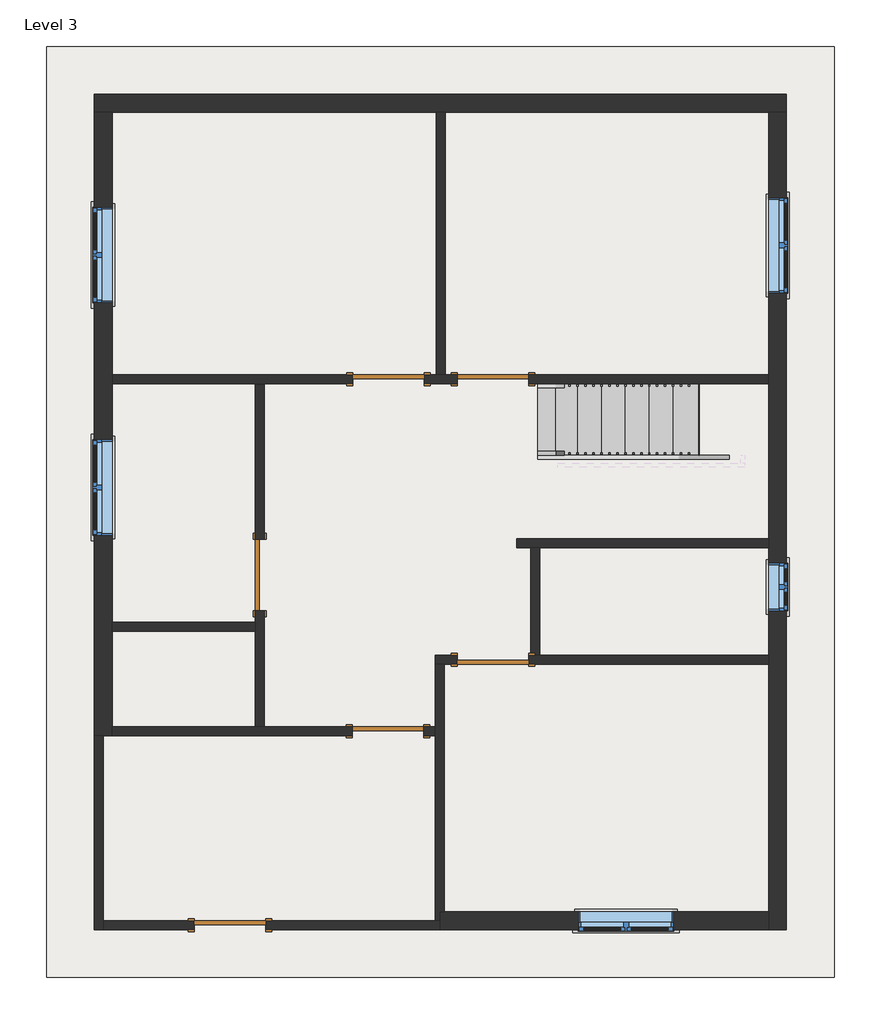
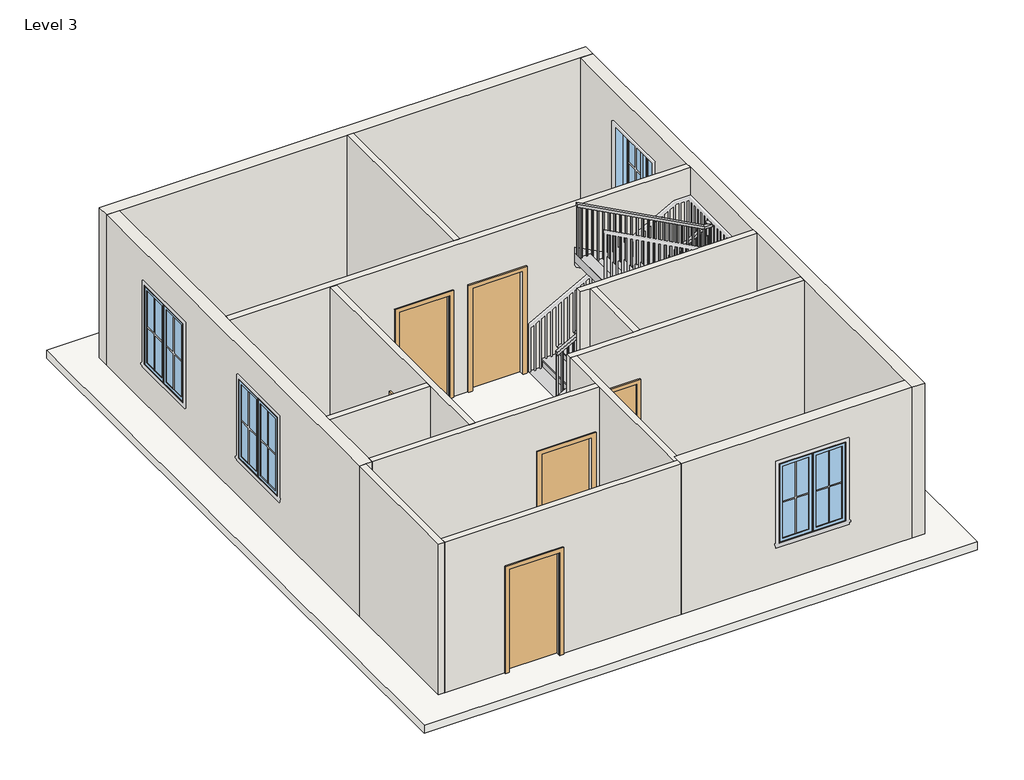
# One storey, part 1 of 2: 15 walls, 6 doors, 5 windows, 1 railing, 1 roof, 1 stair flight.
"""IFC4 building model written with IfcOpenShell, lengths in millimetres."""

from ifc_helpers import new_model, si_unit, frame, origin, place, context, project, spatial, polyline, outline, extrude, faceted_brep, transform, mapped, element, save
from components import door_305aa2a5, door_e5f9f3c4, stair_flight_a6cfe23b, window_c417fced, window_8377141f

model = new_model("IFC4")

# Units and contexts
model_context = context("Model", 3, world=origin())
ifc_project = project(units=[si_unit("LENGTHUNIT", "METRE", prefix="MILLI")], contexts=[model_context])

# Site, building, storey
site = spatial("IfcSite", under=ifc_project)
building = spatial("IfcBuilding", under=site)
storey = spatial("IfcBuildingStorey", under=building, Name="Level 3", Elevation=6096.0)

# Doors
placement = place(None, origin())
door_shape = door_305aa2a5(model_context)
element("IfcDoor", 1, ObjectType="Single-Flush : 36\" x 84\"", at=placement, inside=storey, context=model_context, shape_type="MappedRepresentation", body=[
    mapped(door_shape, transform((8001.0, 9251.95, 6096.0), x_axis=(-1.0, 0.0, 0.0), y_axis=(0.0, -1.0, 0.0), z_axis=(0.0, 0.0, 1.0))),
])
element("IfcDoor", 2, ObjectType="Single-Flush : 36\" x 84\"", at=placement, inside=storey, context=model_context, shape_type="MappedRepresentation", body=[
    mapped(door_shape, transform((5022.9818578, 6750.05, 6096.0), x_axis=(0.0, -1.0, 0.0), y_axis=(1.0, 0.0, 0.0), z_axis=(0.0, 0.0, 1.0))),
])
door_2_shape = door_e5f9f3c4(model_context)
element("IfcDoor", 3, ObjectType="Single-Flush : 36\" x 84\"", at=placement, inside=storey, context=model_context, shape_type="MappedRepresentation", body=[
    mapped(door_2_shape, transform((6667.5, 9251.95, 6096.0), x_axis=(1.0, 0.0, 0.0), y_axis=(0.0, 1.0, 0.0), z_axis=(0.0, 0.0, 1.0))),
])
element("IfcDoor", 4, ObjectType="Single-Flush : 36\" x 84\"", at=placement, inside=storey, context=model_context, shape_type="MappedRepresentation", body=[
    mapped(door_2_shape, transform((8001.0, 5670.55, 6096.0), x_axis=(-1.0, 0.0, 0.0), y_axis=(0.0, -1.0, 0.0), z_axis=(0.0, 0.0, 1.0))),
])
element("IfcDoor", 5, ObjectType="Single-Flush : 36\" x 84\"", at=placement, inside=storey, context=model_context, shape_type="MappedRepresentation", body=[
    mapped(door_2_shape, transform((6658.76875, 4756.15, 6096.0), x_axis=(1.0, 0.0, 0.0), y_axis=(0.0, 1.0, 0.0), z_axis=(0.0, 0.0, 1.0))),
])
element("IfcDoor", 6, ObjectType="Single-Flush : 36\" x 84\"", at=placement, inside=storey, context=model_context, shape_type="MappedRepresentation", body=[
    mapped(door_2_shape, transform((4641.85, 2279.65, 6096.0), x_axis=(1.0, 0.0, 0.0), y_axis=(0.0, 1.0, 0.0), z_axis=(0.0, 0.0, 1.0))),
])

# Railing
element("IfcRailing", 7, ObjectType="Handrail - Rectangular", at=placement, inside=storey, context=model_context, shape_type="SolidModel", body=[
    faceted_brep([(8572.5, 8331.2, 7170.8210526), (8572.5, 8331.2, 7112.9285199), (8572.5, 8280.4, 7112.9285199), (8572.5, 8280.4, 7170.8210526), (11137.9, 8331.2, 8572.962753), (11188.7, 8331.2, 8542.8354025), (11188.7, 8280.4, 8542.8354025), (11137.9, 8280.4, 8572.962753), (11137.9, 8331.2, 8614.6105263), (11188.7, 8331.2, 8563.8105263), (11188.7, 8280.4, 8563.8105263), (11137.9, 8280.4, 8614.6105263), (11264.9, 8331.2, 8614.6105263), (11264.9, 8331.2, 8563.8105263), (11214.1, 8280.4, 8563.8105263), (11214.1, 8280.4, 8614.6105263), (11264.9, 8204.2, 8614.6105263), (11264.9, 8153.4, 8563.8105263), (11214.1, 8153.4, 8563.8105263), (11214.1, 8204.2, 8614.6105263), (11264.9, 8204.2, 8815.9901456), (11264.9, 8153.4, 8765.1901456), (11214.1, 8153.4, 8765.1901456), (11214.1, 8204.2, 8815.9901456), (11264.9, 8077.2, 8815.9901456), (11264.9, 8077.2, 8765.1901456), (11214.1, 8128.0, 8765.1901456), (11214.1, 8128.0, 8815.9901456), (11137.9, 8077.2, 8815.9901456), (11125.1122768, 8077.2, 8765.1901456), (11125.1122768, 8128.0, 8765.1901456), (11137.9, 8128.0, 8815.9901456), (8826.5, 8077.2, 10058.4), (8826.5, 8128.0, 10058.4), (8826.5, 8128.0, 10000.7264198), (8826.5, 8077.2, 10000.7264198)], [[[0, 1, 2, 3]], [[1, 0, 4, 5]], [[2, 1, 5, 6]], [[3, 2, 6, 7]], [[0, 3, 7, 4]], [[5, 4, 8, 9]], [[6, 5, 9, 10]], [[7, 6, 10, 11]], [[4, 7, 11, 8]], [[9, 8, 12, 13]], [[10, 9, 13, 14]], [[11, 10, 14, 15]], [[8, 11, 15, 12]], [[13, 12, 16, 17]], [[14, 13, 17, 18]], [[15, 14, 18, 19]], [[12, 15, 19, 16]], [[17, 16, 20, 21]], [[18, 17, 21, 22]], [[19, 18, 22, 23]], [[16, 19, 23, 20]], [[21, 20, 24, 25]], [[22, 21, 25, 26]], [[23, 22, 26, 27]], [[20, 23, 27, 24]], [[25, 24, 28, 29]], [[26, 25, 29, 30]], [[27, 26, 30, 31]], [[24, 27, 31, 28]], [[32, 33, 34, 35]], [[29, 28, 32, 35]], [[30, 29, 35, 34]], [[31, 30, 34, 33]], [[28, 31, 33, 32]]]),
    extrude(outline(polyline([(9954.6480323, 8912.225), (9964.887674, 8893.175), (8983.5789474, 8893.175), (8983.5789474, 8912.225), (9954.6480323, 8912.225)])), frame((0.0, 8093.075, 0.0), z_axis=(0.0, 1.0, 0.0), x_axis=(0.0, 0.0, 1.0)), (0.0, 0.0, 1.0), 19.05),
    extrude(outline(polyline([(9900.0366101, 9013.825), (9910.2762518, 8994.775), (8983.5789474, 8994.775), (8983.5789474, 9013.825), (9900.0366101, 9013.825)])), frame((0.0, 8093.075, 0.0), z_axis=(0.0, 1.0, 0.0), x_axis=(0.0, 0.0, 1.0)), (0.0, 0.0, 1.0), 19.05),
    extrude(outline(polyline([(9845.425188, 9115.425), (9855.6648296, 9096.375), (8823.1578947, 9096.375), (8823.1578947, 9115.425), (9845.425188, 9115.425)])), frame((0.0, 8093.075, 0.0), z_axis=(0.0, 1.0, 0.0), x_axis=(0.0, 0.0, 1.0)), (0.0, 0.0, 1.0), 19.05),
    extrude(outline(polyline([(9790.8137658, 9217.025), (9801.0534074, 9197.975), (8823.1578947, 9197.975), (8823.1578947, 9217.025), (9790.8137658, 9217.025)])), frame((0.0, 8093.075, 0.0), z_axis=(0.0, 1.0, 0.0), x_axis=(0.0, 0.0, 1.0)), (0.0, 0.0, 1.0), 19.05),
    extrude(outline(polyline([(9736.1597952, 9318.625), (9746.5717386, 9299.575), (8823.1578947, 9299.575), (8823.1578947, 9318.625), (9736.1597952, 9318.625)])), frame((0.0, 8093.075, 0.0), z_axis=(0.0, 1.0, 0.0), x_axis=(0.0, 0.0, 1.0)), (0.0, 0.0, 1.0), 19.05),
    extrude(outline(polyline([(9681.5909214, 9420.225), (9691.8305631, 9401.175), (8662.7368421, 9401.175), (8662.7368421, 9420.225), (9681.5909214, 9420.225)])), frame((0.0, 8093.075, 0.0), z_axis=(0.0, 1.0, 0.0), x_axis=(0.0, 0.0, 1.0)), (0.0, 0.0, 1.0), 19.05),
    extrude(outline(polyline([(9626.9794993, 9521.825), (9637.2191409, 9502.775), (8662.7368421, 9502.775), (8662.7368421, 9521.825), (9626.9794993, 9521.825)])), frame((0.0, 8093.075, 0.0), z_axis=(0.0, 1.0, 0.0), x_axis=(0.0, 0.0, 1.0)), (0.0, 0.0, 1.0), 19.05),
    extrude(outline(polyline([(9572.3680771, 9623.425), (9582.6077187, 9604.375), (8662.7368421, 9604.375), (8662.7368421, 9623.425), (9572.3680771, 9623.425)])), frame((0.0, 8093.075, 0.0), z_axis=(0.0, 1.0, 0.0), x_axis=(0.0, 0.0, 1.0)), (0.0, 0.0, 1.0), 19.05),
    extrude(outline(polyline([(9517.7566549, 9725.025), (9527.9962966, 9705.975), (8502.3157895, 9705.975), (8502.3157895, 9725.025), (9517.7566549, 9725.025)])), frame((0.0, 8093.075, 0.0), z_axis=(0.0, 1.0, 0.0), x_axis=(0.0, 0.0, 1.0)), (0.0, 0.0, 1.0), 19.05),
    extrude(outline(polyline([(9463.1452327, 9826.625), (9473.3848744, 9807.575), (8502.3157895, 9807.575), (8502.3157895, 9826.625), (9463.1452327, 9826.625)])), frame((0.0, 8093.075, 0.0), z_axis=(0.0, 1.0, 0.0), x_axis=(0.0, 0.0, 1.0)), (0.0, 0.0, 1.0), 19.05),
    extrude(outline(polyline([(9408.5338106, 9928.225), (9418.7734522, 9909.175), (8502.3157895, 9909.175), (8502.3157895, 9928.225), (9408.5338106, 9928.225)])), frame((0.0, 8093.075, 0.0), z_axis=(0.0, 1.0, 0.0), x_axis=(0.0, 0.0, 1.0)), (0.0, 0.0, 1.0), 19.05),
    extrude(outline(polyline([(9353.9223884, 10029.825), (9364.1620301, 10010.775), (8341.8947368, 10010.775), (8341.8947368, 10029.825), (9353.9223884, 10029.825)])), frame((0.0, 8093.075, 0.0), z_axis=(0.0, 1.0, 0.0), x_axis=(0.0, 0.0, 1.0)), (0.0, 0.0, 1.0), 19.05),
    extrude(outline(polyline([(9299.3109662, 10131.425), (9309.5506079, 10112.375), (8341.8947368, 10112.375), (8341.8947368, 10131.425), (9299.3109662, 10131.425)])), frame((0.0, 8093.075, 0.0), z_axis=(0.0, 1.0, 0.0), x_axis=(0.0, 0.0, 1.0)), (0.0, 0.0, 1.0), 19.05),
    extrude(outline(polyline([(9244.6995441, 10233.025), (9254.9391857, 10213.975), (8341.8947368, 10213.975), (8341.8947368, 10233.025), (9244.6995441, 10233.025)])), frame((0.0, 8093.075, 0.0), z_axis=(0.0, 1.0, 0.0), x_axis=(0.0, 0.0, 1.0)), (0.0, 0.0, 1.0), 19.05),
    extrude(outline(polyline([(9190.0881219, 10334.625), (9200.3277635, 10315.575), (8181.4736842, 10315.575), (8181.4736842, 10334.625), (9190.0881219, 10334.625)])), frame((0.0, 8093.075, 0.0), z_axis=(0.0, 1.0, 0.0), x_axis=(0.0, 0.0, 1.0)), (0.0, 0.0, 1.0), 19.05),
    extrude(outline(polyline([(9135.4766997, 10436.225), (9145.7163414, 10417.175), (8181.4736842, 10417.175), (8181.4736842, 10436.225), (9135.4766997, 10436.225)])), frame((0.0, 8093.075, 0.0), z_axis=(0.0, 1.0, 0.0), x_axis=(0.0, 0.0, 1.0)), (0.0, 0.0, 1.0), 19.05),
    extrude(outline(polyline([(9080.8652775, 10537.825), (9091.1049192, 10518.775), (8181.4736842, 10518.775), (8181.4736842, 10537.825), (9080.8652775, 10537.825)])), frame((0.0, 8093.075, 0.0), z_axis=(0.0, 1.0, 0.0), x_axis=(0.0, 0.0, 1.0)), (0.0, 0.0, 1.0), 19.05),
    extrude(outline(polyline([(9026.2538554, 10639.425), (9036.493497, 10620.375), (8021.0526316, 10620.375), (8021.0526316, 10639.425), (9026.2538554, 10639.425)])), frame((0.0, 8093.075, 0.0), z_axis=(0.0, 1.0, 0.0), x_axis=(0.0, 0.0, 1.0)), (0.0, 0.0, 1.0), 19.05),
    extrude(outline(polyline([(8971.6424332, 10741.025), (8981.8820749, 10721.975), (8021.0526316, 10721.975), (8021.0526316, 10741.025), (8971.6424332, 10741.025)])), frame((0.0, 8093.075, 0.0), z_axis=(0.0, 1.0, 0.0), x_axis=(0.0, 0.0, 1.0)), (0.0, 0.0, 1.0), 19.05),
    extrude(outline(polyline([(8917.031011, 10842.625), (8927.2706527, 10823.575), (8021.0526316, 10823.575), (8021.0526316, 10842.625), (8917.031011, 10842.625)])), frame((0.0, 8093.075, 0.0), z_axis=(0.0, 1.0, 0.0), x_axis=(0.0, 0.0, 1.0)), (0.0, 0.0, 1.0), 19.05),
    extrude(outline(polyline([(8862.4195889, 10944.225), (8872.6592305, 10925.175), (7860.6315789, 10925.175), (7860.6315789, 10944.225), (8862.4195889, 10944.225)])), frame((0.0, 8093.075, 0.0), z_axis=(0.0, 1.0, 0.0), x_axis=(0.0, 0.0, 1.0)), (0.0, 0.0, 1.0), 19.05),
    extrude(outline(polyline([(8807.8081667, 11045.825), (8818.0478083, 11026.775), (7860.6315789, 11026.775), (7860.6315789, 11045.825), (8807.8081667, 11045.825)])), frame((0.0, 8093.075, 0.0), z_axis=(0.0, 1.0, 0.0), x_axis=(0.0, 0.0, 1.0)), (0.0, 0.0, 1.0), 19.05),
    extrude(outline(polyline([(8753.1967445, 11147.425), (8763.4363862, 11128.375), (7860.6315789, 11128.375), (7860.6315789, 11147.425), (8753.1967445, 11147.425)])), frame((0.0, 8093.075, 0.0), z_axis=(0.0, 1.0, 0.0), x_axis=(0.0, 0.0, 1.0)), (0.0, 0.0, 1.0), 19.05),
    extrude(outline(polyline([(11229.975, 8213.725), (11249.025, 8213.725), (11249.025, 8194.675), (11229.975, 8194.675), (11229.975, 8213.725)])), frame((0.0, 0.0, 7700.2105263), z_axis=(0.0, 0.0, 1.0), x_axis=(1.0, 0.0, 0.0)), (0.0, 0.0, 1.0), 863.6),
    extrude(outline(polyline([(11204.575, 8296.275), (11204.575, 8315.325), (11223.625, 8315.325), (11223.625, 8296.275), (11204.575, 8296.275)])), frame((0.0, 0.0, 7700.2105263), z_axis=(0.0, 0.0, 1.0), x_axis=(1.0, 0.0, 0.0)), (0.0, 0.0, 1.0), 863.6),
    extrude(outline(polyline([(8506.3936009, 11122.025), (8495.9816576, 11102.975), (7539.7894737, 11102.975), (7539.7894737, 11122.025), (8506.3936009, 11122.025)])), frame((0.0, 8296.275, 0.0), z_axis=(0.0, 1.0, 0.0), x_axis=(0.0, 0.0, 1.0)), (0.0, 0.0, 1.0), 19.05),
    extrude(outline(polyline([(8450.8632365, 11020.425), (8440.4512932, 11001.375), (7539.7894737, 11001.375), (7539.7894737, 11020.425), (8450.8632365, 11020.425)])), frame((0.0, 8296.275, 0.0), z_axis=(0.0, 1.0, 0.0), x_axis=(0.0, 0.0, 1.0)), (0.0, 0.0, 1.0), 19.05),
    extrude(outline(polyline([(8395.3328722, 10918.825), (8384.9209288, 10899.775), (7539.7894737, 10899.775), (7539.7894737, 10918.825), (8395.3328722, 10918.825)])), frame((0.0, 8296.275, 0.0), z_axis=(0.0, 1.0, 0.0), x_axis=(0.0, 0.0, 1.0)), (0.0, 0.0, 1.0), 19.05),
    extrude(outline(polyline([(8339.8025078, 10817.225), (8329.3905645, 10798.175), (7379.3684211, 10798.175), (7379.3684211, 10817.225), (8339.8025078, 10817.225)])), frame((0.0, 8296.275, 0.0), z_axis=(0.0, 1.0, 0.0), x_axis=(0.0, 0.0, 1.0)), (0.0, 0.0, 1.0), 19.05),
    extrude(outline(polyline([(8284.2721434, 10715.625), (8273.8602001, 10696.575), (7379.3684211, 10696.575), (7379.3684211, 10715.625), (8284.2721434, 10715.625)])), frame((0.0, 8296.275, 0.0), z_axis=(0.0, 1.0, 0.0), x_axis=(0.0, 0.0, 1.0)), (0.0, 0.0, 1.0), 19.05),
    extrude(outline(polyline([(8228.741779, 10614.025), (8218.3298357, 10594.975), (7379.3684211, 10594.975), (7379.3684211, 10614.025), (8228.741779, 10614.025)])), frame((0.0, 8296.275, 0.0), z_axis=(0.0, 1.0, 0.0), x_axis=(0.0, 0.0, 1.0)), (0.0, 0.0, 1.0), 19.05),
    extrude(outline(polyline([(8173.2114147, 10512.425), (8162.7994714, 10493.375), (7218.9473684, 10493.375), (7218.9473684, 10512.425), (8173.2114147, 10512.425)])), frame((0.0, 8296.275, 0.0), z_axis=(0.0, 1.0, 0.0), x_axis=(0.0, 0.0, 1.0)), (0.0, 0.0, 1.0), 19.05),
    extrude(outline(polyline([(8117.6810503, 10410.825), (8107.269107, 10391.775), (7218.9473684, 10391.775), (7218.9473684, 10410.825), (8117.6810503, 10410.825)])), frame((0.0, 8296.275, 0.0), z_axis=(0.0, 1.0, 0.0), x_axis=(0.0, 0.0, 1.0)), (0.0, 0.0, 1.0), 19.05),
    extrude(outline(polyline([(8062.1506859, 10309.225), (8051.7387426, 10290.175), (7218.9473684, 10290.175), (7218.9473684, 10309.225), (8062.1506859, 10309.225)])), frame((0.0, 8296.275, 0.0), z_axis=(0.0, 1.0, 0.0), x_axis=(0.0, 0.0, 1.0)), (0.0, 0.0, 1.0), 19.05),
    extrude(outline(polyline([(8006.6203216, 10207.625), (7996.2083782, 10188.575), (7058.5263158, 10188.575), (7058.5263158, 10207.625), (8006.6203216, 10207.625)])), frame((0.0, 8296.275, 0.0), z_axis=(0.0, 1.0, 0.0), x_axis=(0.0, 0.0, 1.0)), (0.0, 0.0, 1.0), 19.05),
    extrude(outline(polyline([(7951.0899572, 10106.025), (7940.6780139, 10086.975), (7058.5263158, 10086.975), (7058.5263158, 10106.025), (7951.0899572, 10106.025)])), frame((0.0, 8296.275, 0.0), z_axis=(0.0, 1.0, 0.0), x_axis=(0.0, 0.0, 1.0)), (0.0, 0.0, 1.0), 19.05),
    extrude(outline(polyline([(7895.5595928, 10004.425), (7885.1476495, 9985.375), (7058.5263158, 9985.375), (7058.5263158, 10004.425), (7895.5595928, 10004.425)])), frame((0.0, 8296.275, 0.0), z_axis=(0.0, 1.0, 0.0), x_axis=(0.0, 0.0, 1.0)), (0.0, 0.0, 1.0), 19.05),
    extrude(outline(polyline([(7840.0292284, 9902.825), (7829.6172851, 9883.775), (6898.1052632, 9883.775), (6898.1052632, 9902.825), (7840.0292284, 9902.825)])), frame((0.0, 8296.275, 0.0), z_axis=(0.0, 1.0, 0.0), x_axis=(0.0, 0.0, 1.0)), (0.0, 0.0, 1.0), 19.05),
    extrude(outline(polyline([(7784.4988641, 9801.225), (7774.0869207, 9782.175), (6898.1052632, 9782.175), (6898.1052632, 9801.225), (7784.4988641, 9801.225)])), frame((0.0, 8296.275, 0.0), z_axis=(0.0, 1.0, 0.0), x_axis=(0.0, 0.0, 1.0)), (0.0, 0.0, 1.0), 19.05),
    extrude(outline(polyline([(7728.9684997, 9699.625), (7718.5565564, 9680.575), (6898.1052632, 9680.575), (6898.1052632, 9699.625), (7728.9684997, 9699.625)])), frame((0.0, 8296.275, 0.0), z_axis=(0.0, 1.0, 0.0), x_axis=(0.0, 0.0, 1.0)), (0.0, 0.0, 1.0), 19.05),
    extrude(outline(polyline([(7673.4381353, 9598.025), (7663.026192, 9578.975), (6737.6842105, 9578.975), (6737.6842105, 9598.025), (7673.4381353, 9598.025)])), frame((0.0, 8296.275, 0.0), z_axis=(0.0, 1.0, 0.0), x_axis=(0.0, 0.0, 1.0)), (0.0, 0.0, 1.0), 19.05),
    extrude(outline(polyline([(7617.9077709, 9496.425), (7607.4958276, 9477.375), (6737.6842105, 9477.375), (6737.6842105, 9496.425), (7617.9077709, 9496.425)])), frame((0.0, 8296.275, 0.0), z_axis=(0.0, 1.0, 0.0), x_axis=(0.0, 0.0, 1.0)), (0.0, 0.0, 1.0), 19.05),
    extrude(outline(polyline([(7562.3774066, 9394.825), (7551.9654633, 9375.775), (6737.6842105, 9375.775), (6737.6842105, 9394.825), (7562.3774066, 9394.825)])), frame((0.0, 8296.275, 0.0), z_axis=(0.0, 1.0, 0.0), x_axis=(0.0, 0.0, 1.0)), (0.0, 0.0, 1.0), 19.05),
    extrude(outline(polyline([(7506.8470422, 9293.225), (7496.4350989, 9274.175), (6577.2631579, 9274.175), (6577.2631579, 9293.225), (7506.8470422, 9293.225)])), frame((0.0, 8296.275, 0.0), z_axis=(0.0, 1.0, 0.0), x_axis=(0.0, 0.0, 1.0)), (0.0, 0.0, 1.0), 19.05),
    extrude(outline(polyline([(7451.3166778, 9191.625), (7440.9047345, 9172.575), (6577.2631579, 9172.575), (6577.2631579, 9191.625), (7451.3166778, 9191.625)])), frame((0.0, 8296.275, 0.0), z_axis=(0.0, 1.0, 0.0), x_axis=(0.0, 0.0, 1.0)), (0.0, 0.0, 1.0), 19.05),
    extrude(outline(polyline([(7395.7863135, 9090.025), (7385.3743701, 9070.975), (6577.2631579, 9070.975), (6577.2631579, 9090.025), (7395.7863135, 9090.025)])), frame((0.0, 8296.275, 0.0), z_axis=(0.0, 1.0, 0.0), x_axis=(0.0, 0.0, 1.0)), (0.0, 0.0, 1.0), 19.05),
    extrude(outline(polyline([(7340.2559491, 8988.425), (7329.8440058, 8969.375), (6416.8421053, 8969.375), (6416.8421053, 8988.425), (7340.2559491, 8988.425)])), frame((0.0, 8296.275, 0.0), z_axis=(0.0, 1.0, 0.0), x_axis=(0.0, 0.0, 1.0)), (0.0, 0.0, 1.0), 19.05),
    extrude(outline(polyline([(7284.7255847, 8886.825), (7274.3136414, 8867.775), (6416.8421053, 8867.775), (6416.8421053, 8886.825), (7284.7255847, 8886.825)])), frame((0.0, 8296.275, 0.0), z_axis=(0.0, 1.0, 0.0), x_axis=(0.0, 0.0, 1.0)), (0.0, 0.0, 1.0), 19.05),
    extrude(outline(polyline([(7229.1952203, 8785.225), (7218.783277, 8766.175), (6256.4210526, 8766.175), (6256.4210526, 8785.225), (7229.1952203, 8785.225)])), frame((0.0, 8296.275, 0.0), z_axis=(0.0, 1.0, 0.0), x_axis=(0.0, 0.0, 1.0)), (0.0, 0.0, 1.0), 19.05),
    extrude(outline(polyline([(7173.664856, 8683.625), (7163.2529126, 8664.575), (6256.4210526, 8664.575), (6256.4210526, 8683.625), (7173.664856, 8683.625)])), frame((0.0, 8296.275, 0.0), z_axis=(0.0, 1.0, 0.0), x_axis=(0.0, 0.0, 1.0)), (0.0, 0.0, 1.0), 19.05),
    extrude(outline(polyline([(11229.975, 8112.125), (11249.025, 8112.125), (11249.025, 8093.075), (11229.975, 8093.075), (11229.975, 8112.125)])), frame((0.0, 0.0, 7700.2105263), z_axis=(0.0, 0.0, 1.0), x_axis=(1.0, 0.0, 0.0)), (0.0, 0.0, 1.0), 1064.9796193),
    extrude(outline(polyline([(11229.975, 8296.275), (11229.975, 8315.325), (11249.025, 8315.325), (11249.025, 8296.275), (11229.975, 8296.275)])), frame((0.0, 0.0, 7700.2105263), z_axis=(0.0, 0.0, 1.0), x_axis=(1.0, 0.0, 0.0)), (0.0, 0.0, 1.0), 863.6),
    extrude(outline(polyline([(9990.4867781, 8845.55), (10000.7264198, 8826.5), (8983.5789474, 8826.5), (8983.5789474, 8845.55), (9990.4867781, 8845.55)])), frame((0.0, 8093.075, 0.0), z_axis=(0.0, 1.0, 0.0), x_axis=(0.0, 0.0, 1.0)), (0.0, 0.0, 1.0), 19.05),
    extrude(outline(polyline([(7123.3404633, 8591.55), (7112.9285199, 8572.5), (6256.4210526, 8572.5), (6256.4210526, 8591.55), (7123.3404633, 8591.55)])), frame((0.0, 8296.275, 0.0), z_axis=(0.0, 1.0, 0.0), x_axis=(0.0, 0.0, 1.0)), (0.0, 0.0, 1.0), 19.05),
])

# Roof
element("IfcRoof", 8, ObjectType="Generic - 12\"", at=placement, inside=storey, context=model_context, shape_type="SweptSolid", body=[
    extrude(outline(polyline([(2298.7, 13500.1), (12357.1, 13500.1), (12357.1, 1612.9), (2298.7, 1612.9), (2298.7, 13500.1)])), frame((0.0, 0.0, 6096.0), z_axis=(0.0, 0.0, 1.0), x_axis=(1.0, 0.0, 0.0)), (0.0, 0.0, 1.0), 152.4),
])

# Stair flight
stair_flight_shape = stair_flight_a6cfe23b(model_context)
element("IfcStairFlight", 9, ObjectType="2\" Tread 1\" Nosing 1/4\" Riser", at=placement, inside=storey, context=model_context, shape_type="MappedRepresentation", body=[
    mapped(stair_flight_shape, transform((0.0, 0.0, 0.0), x_axis=(1.0, 0.0, 0.0), y_axis=(0.0, 1.0, 0.0), z_axis=(0.0, 0.0, 1.0))),
])

# Walls
element("IfcWall", 10, ObjectType="Generic - 5\"", at=placement, inside=storey, context=model_context, shape_type="Brep", body=[
    faceted_brep([(7115.96875, 4699.0, 8229.6), (7115.96875, 4699.0, 6096.0), (7264.4, 4699.0, 6096.0), (7264.4, 4699.0, 9144.0), (3136.9, 4699.0, 9144.0), (3136.9, 4699.0, 6096.0), (6201.56875, 4699.0, 6096.0), (6201.56875, 4699.0, 8229.6), (7264.4, 4813.3, 6096.0), (7115.96875, 4813.3, 6096.0), (7115.96875, 4813.3, 8229.6), (6201.56875, 4813.3, 8229.6), (6201.56875, 4813.3, 6096.0), (5080.1318578, 4813.3, 6096.0), (4965.8318578, 4813.3, 6096.0), (3136.9, 4813.3, 6096.0), (3136.9, 4813.3, 9144.0), (4965.8318578, 4813.3, 9144.0), (5080.1318578, 4813.3, 9144.0), (7264.4, 4813.3, 9144.0)], [[[0, 1, 2, 3, 4, 5, 6, 7]], [[8, 9, 10, 11, 12, 13, 14, 15, 16, 17, 18, 19]], [[6, 5, 15, 14, 13, 12]], [[2, 1, 9, 8]], [[4, 3, 19, 18, 17, 16]], [[5, 4, 16, 15]], [[3, 2, 8, 19]], [[10, 9, 1, 0]], [[11, 10, 0, 7]], [[12, 11, 7, 6]]]),
])
element("IfcWall", 11, ObjectType="Generic - 5\"", at=placement, inside=storey, context=model_context, shape_type="SweptSolid", body=[
    extrude(outline(polyline([(4965.8318578, 6032.5), (3136.9, 6032.5), (3136.9, 6146.8), (4965.8318578, 6146.8), (4965.8318578, 6032.5)])), frame((0.0, 0.0, 6096.0), z_axis=(0.0, 0.0, 1.0), x_axis=(1.0, 0.0, 0.0)), (0.0, 0.0, 1.0), 3048.0),
])
element("IfcWall", 12, ObjectType="Generic - 5\"", at=placement, inside=storey, context=model_context, shape_type="Brep", body=[
    faceted_brep([(5080.1318578, 4813.3, 6096.0), (5080.1318578, 6292.85, 6096.0), (5080.1318578, 6292.85, 8229.6), (5080.1318578, 7207.25, 8229.6), (5080.1318578, 7207.25, 6096.0), (5080.1318578, 9182.1, 6096.0), (5080.1318578, 9182.1, 9144.0), (5080.1318578, 4813.3, 9144.0), (4965.8318578, 6292.85, 8229.6), (4965.8318578, 6292.85, 6096.0), (4965.8318578, 6146.8, 6096.0), (4965.8318578, 6032.5, 6096.0), (4965.8318578, 4813.3, 6096.0), (4965.8318578, 4813.3, 9144.0), (4965.8318578, 6032.5, 9144.0), (4965.8318578, 6146.8, 9144.0), (4965.8318578, 9182.1, 9144.0), (4965.8318578, 9182.1, 6096.0), (4965.8318578, 7207.25, 6096.0), (4965.8318578, 7207.25, 8229.6)], [[[0, 1, 2, 3, 4, 5, 6, 7]], [[8, 9, 10, 11, 12, 13, 14, 15, 16, 17, 18, 19]], [[18, 17, 5, 4]], [[12, 11, 10, 9, 1, 0]], [[6, 5, 17, 16]], [[7, 6, 16, 15, 14, 13]], [[0, 7, 13, 12]], [[2, 1, 9, 8]], [[3, 2, 8, 19]], [[4, 3, 19, 18]]]),
])
element("IfcWall", 13, ObjectType="Generic - 5\"", at=placement, inside=storey, context=model_context, shape_type="Brep", body=[
    faceted_brep([(7124.7, 9194.8, 8229.6), (7124.7, 9194.8, 6096.0), (7543.8, 9194.8, 6096.0), (7543.8, 9194.8, 8229.6), (8458.2, 9194.8, 8229.6), (8458.2, 9194.8, 6096.0), (11518.9, 9194.8, 6096.0), (11518.9, 9194.8, 9144.0), (3136.9, 9194.8, 9144.0), (3136.9, 9194.8, 6096.0), (6210.3, 9194.8, 6096.0), (6210.3, 9194.8, 8229.6), (7543.8, 9309.1, 6096.0), (7391.4, 9309.1, 6096.0), (7277.1, 9309.1, 6096.0), (7124.7, 9309.1, 6096.0), (7124.7, 9309.1, 8229.6), (6210.3, 9309.1, 8229.6), (6210.3, 9309.1, 6096.0), (3136.9, 9309.1, 6096.0), (3136.9, 9309.1, 9144.0), (7277.1, 9309.1, 9144.0), (7391.4, 9309.1, 9144.0), (11518.9, 9309.1, 9144.0), (11518.9, 9309.1, 6096.0), (8458.2, 9309.1, 6096.0), (8458.2, 9309.1, 8229.6), (7543.8, 9309.1, 8229.6)], [[[0, 1, 2, 3, 4, 5, 6, 7, 8, 9, 10, 11]], [[12, 13, 14, 15, 16, 17, 18, 19, 20, 21, 22, 23, 24, 25, 26, 27]], [[25, 24, 6, 5]], [[10, 9, 19, 18]], [[2, 1, 15, 14, 13, 12]], [[8, 7, 23, 22, 21, 20]], [[7, 6, 24, 23]], [[9, 8, 20, 19]], [[3, 2, 12, 27]], [[4, 3, 27, 26]], [[5, 4, 26, 25]], [[16, 15, 1, 0]], [[17, 16, 0, 11]], [[18, 17, 11, 10]]]),
])
element("IfcWall", 14, ObjectType="Generic - 5\"", at=placement, inside=storey, context=model_context, shape_type="SweptSolid", body=[
    extrude(outline(polyline([(7277.1, 9309.1), (7277.1, 12661.9), (7391.4, 12661.9), (7391.4, 9309.1), (7277.1, 9309.1)])), frame((0.0, 0.0, 6096.0), z_axis=(0.0, 0.0, 1.0), x_axis=(1.0, 0.0, 0.0)), (0.0, 0.0, 1.0), 3048.0),
])
element("IfcWall", 15, ObjectType="Generic - 5\"", at=placement, inside=storey, context=model_context, shape_type="Brep", body=[
    faceted_brep([(2908.3, 4699.0, 6096.0), (2908.3, 2222.5, 6096.0), (2908.3, 2222.5, 9144.0), (2908.3, 4699.0, 9144.0), (3022.6, 4699.0, 6096.0), (3022.6, 4699.0, 9144.0), (3022.6, 2336.8, 9144.0), (3022.6, 2222.5, 9144.0), (3022.6, 2222.5, 6096.0), (3022.6, 2336.8, 6096.0)], [[[0, 1, 2, 3]], [[4, 5, 6, 7, 8, 9]], [[1, 0, 4, 9, 8]], [[3, 2, 7, 6, 5]], [[0, 3, 5, 4]], [[2, 1, 8, 7]]]),
])
element("IfcWall", 16, ObjectType="Generic - 5\"", at=placement, inside=storey, context=model_context, shape_type="Brep", body=[
    faceted_brep([(5099.05, 2222.5, 8229.6), (5099.05, 2222.5, 6096.0), (7321.55, 2222.5, 6096.0), (7321.55, 2222.5, 9144.0), (3022.6, 2222.5, 9144.0), (3022.6, 2222.5, 6096.0), (4184.65, 2222.5, 6096.0), (4184.65, 2222.5, 8229.6), (7321.55, 2336.8, 6096.0), (7264.4, 2336.8, 6096.0), (5099.05, 2336.8, 6096.0), (5099.05, 2336.8, 8229.6), (4184.65, 2336.8, 8229.6), (4184.65, 2336.8, 6096.0), (3022.6, 2336.8, 6096.0), (3022.6, 2336.8, 9144.0), (7264.4, 2336.8, 9144.0), (7321.55, 2336.8, 9144.0)], [[[0, 1, 2, 3, 4, 5, 6, 7]], [[8, 9, 10, 11, 12, 13, 14, 15, 16, 17]], [[6, 5, 14, 13]], [[2, 1, 10, 9, 8]], [[3, 2, 8, 17]], [[4, 3, 17, 16, 15]], [[5, 4, 15, 14]], [[11, 10, 1, 0]], [[12, 11, 0, 7]], [[13, 12, 7, 6]]]),
])
element("IfcWall", 17, ObjectType="Generic - 5\"", at=placement, inside=storey, context=model_context, shape_type="Brep", body=[
    faceted_brep([(11518.9, 7213.6, 6096.0), (8305.8, 7213.6, 6096.0), (8305.8, 7213.6, 9144.0), (11518.9, 7213.6, 9144.0), (11518.9, 7099.3, 6096.0), (11518.9, 7099.3, 9144.0), (8597.9, 7099.3, 9144.0), (8483.6, 7099.3, 9144.0), (8305.8, 7099.3, 9144.0), (8305.8, 7099.3, 6096.0), (8483.6, 7099.3, 6096.0), (8597.9, 7099.3, 6096.0)], [[[0, 1, 2, 3]], [[4, 5, 6, 7, 8, 9, 10, 11]], [[1, 0, 4, 11, 10, 9]], [[2, 1, 9, 8]], [[3, 2, 8, 7, 6, 5]], [[0, 3, 5, 4]]]),
])
element("IfcWall", 18, ObjectType="Generic - 5\"", at=placement, inside=storey, context=model_context, shape_type="SweptSolid", body=[
    extrude(outline(polyline([(8483.6, 5727.7), (8483.6, 7099.3), (8597.9, 7099.3), (8597.9, 5727.7), (8483.6, 5727.7)])), frame((0.0, 0.0, 6096.0), z_axis=(0.0, 0.0, 1.0), x_axis=(1.0, 0.0, 0.0)), (0.0, 0.0, 1.0), 3048.0),
])
element("IfcWall", 19, ObjectType="Generic - 5\"", at=placement, inside=storey, context=model_context, shape_type="Brep", body=[
    faceted_brep([(7543.8, 5727.7, 8229.6), (7543.8, 5727.7, 6096.0), (7264.4, 5727.7, 6096.0), (7264.4, 5727.7, 9144.0), (8483.6, 5727.7, 9144.0), (8597.9, 5727.7, 9144.0), (11518.9, 5727.7, 9144.0), (11518.9, 5727.7, 6096.0), (8597.9, 5727.7, 6096.0), (8483.6, 5727.7, 6096.0), (8458.2, 5727.7, 6096.0), (8458.2, 5727.7, 8229.6), (7264.4, 5613.4, 6096.0), (7378.7, 5613.4, 6096.0), (7543.8, 5613.4, 6096.0), (7543.8, 5613.4, 8229.6), (8458.2, 5613.4, 8229.6), (8458.2, 5613.4, 6096.0), (11518.9, 5613.4, 6096.0), (11518.9, 5613.4, 9144.0), (7378.7, 5613.4, 9144.0), (7264.4, 5613.4, 9144.0)], [[[0, 1, 2, 3, 4, 5, 6, 7, 8, 9, 10, 11]], [[12, 13, 14, 15, 16, 17, 18, 19, 20, 21]], [[2, 1, 14, 13, 12]], [[10, 9, 8, 7, 18, 17]], [[6, 5, 4, 3, 21, 20, 19]], [[7, 6, 19, 18]], [[3, 2, 12, 21]], [[15, 14, 1, 0]], [[16, 15, 0, 11]], [[17, 16, 11, 10]]]),
])
element("IfcWall", 20, ObjectType="Generic - 5\"", at=placement, inside=storey, context=model_context, shape_type="Brep", body=[
    faceted_brep([(7264.4, 5613.4, 6096.0), (7264.4, 4813.3, 6096.0), (7264.4, 4699.0, 6096.0), (7264.4, 2336.8, 6096.0), (7264.4, 2336.8, 9144.0), (7264.4, 4699.0, 9144.0), (7264.4, 4813.3, 9144.0), (7264.4, 5613.4, 9144.0), (7378.7, 5613.4, 6096.0), (7378.7, 5613.4, 9144.0), (7378.7, 2451.1, 9144.0), (7378.7, 2451.1, 6096.0), (7321.55, 2451.1, 6096.0), (7321.55, 2336.8, 6096.0), (7321.55, 2336.8, 9144.0), (7321.55, 2451.1, 9144.0)], [[[0, 1, 2, 3, 4, 5, 6, 7]], [[8, 9, 10, 11]], [[3, 2, 1, 0, 8, 11, 12, 13]], [[7, 6, 5, 4, 14, 15, 10, 9]], [[0, 7, 9, 8]], [[4, 3, 13, 14]], [[13, 12, 15, 14]], [[12, 11, 10, 15]]]),
])
element("IfcWall", 21, ObjectType="Generic - 8\"", at=placement, inside=storey, context=model_context, shape_type="Brep", body=[
    faceted_brep([(2908.3, 12661.9, 6096.0), (3136.9, 12661.9, 6096.0), (7277.1, 12661.9, 6096.0), (7391.4, 12661.9, 6096.0), (11518.9, 12661.9, 6096.0), (11747.5, 12661.9, 6096.0), (11747.5, 12661.9, 9144.0), (11518.9, 12661.9, 9144.0), (7391.4, 12661.9, 9144.0), (7277.1, 12661.9, 9144.0), (3136.9, 12661.9, 9144.0), (2908.3, 12661.9, 9144.0), (2908.3, 12890.5, 6096.0), (2908.3, 12890.5, 9144.0), (11747.5, 12890.5, 9144.0), (11747.5, 12890.5, 6096.0)], [[[0, 1, 2, 3, 4, 5, 6, 7, 8, 9, 10, 11]], [[12, 13, 14, 15]], [[5, 4, 3, 2, 1, 0, 12, 15]], [[11, 10, 9, 8, 7, 6, 14, 13]], [[6, 5, 15, 14]], [[0, 11, 13, 12]]]),
])
element("IfcWall", 22, ObjectType="Generic - 8\"", at=placement, inside=storey, context=model_context, shape_type="Brep", body=[
    faceted_brep([(11518.9, 12661.9, 6096.0), (11518.9, 9309.1, 6096.0), (11518.9, 9194.8, 6096.0), (11518.9, 7213.6, 6096.0), (11518.9, 7099.3, 6096.0), (11518.9, 5727.7, 6096.0), (11518.9, 5613.4, 6096.0), (11518.9, 2451.1, 6096.0), (11518.9, 2222.5, 6096.0), (11518.9, 2222.5, 9144.0), (11518.9, 2451.1, 9144.0), (11518.9, 5613.4, 9144.0), (11518.9, 5727.7, 9144.0), (11518.9, 7099.3, 9144.0), (11518.9, 7213.6, 9144.0), (11518.9, 9194.8, 9144.0), (11518.9, 9309.1, 9144.0), (11518.9, 12661.9, 9144.0), (11518.9, 10352.0875, 8534.4), (11518.9, 10352.0875, 7010.4), (11518.9, 11571.2875, 7010.4), (11518.9, 11571.2875, 8534.4), (11518.9, 6292.85, 7924.8), (11518.9, 6292.85, 7010.4), (11518.9, 6902.45, 7010.4), (11518.9, 6902.45, 7924.8), (11747.5, 12661.9, 6096.0), (11747.5, 12661.9, 9144.0), (11747.5, 2222.5, 9144.0), (11747.5, 2222.5, 6096.0), (11747.5, 10352.0875, 8534.4), (11747.5, 11571.2875, 8534.4), (11747.5, 11571.2875, 7010.4), (11747.5, 10352.0875, 7010.4), (11747.5, 6292.85, 7924.8), (11747.5, 6902.45, 7924.8), (11747.5, 6902.45, 7010.4), (11747.5, 6292.85, 7010.4)], [[[0, 1, 2, 3, 4, 5, 6, 7, 8, 9, 10, 11, 12, 13, 14, 15, 16, 17], [18, 19, 20, 21], [22, 23, 24, 25]], [[26, 27, 28, 29], [30, 31, 32, 33], [34, 35, 36, 37]], [[8, 7, 6, 5, 4, 3, 2, 1, 0, 26, 29]], [[17, 16, 15, 14, 13, 12, 11, 10, 9, 28, 27]], [[0, 17, 27, 26]], [[9, 8, 29, 28]], [[19, 18, 30, 33]], [[20, 19, 33, 32]], [[21, 20, 32, 31]], [[18, 21, 31, 30]], [[23, 22, 34, 37]], [[24, 23, 37, 36]], [[25, 24, 36, 35]], [[22, 25, 35, 34]]]),
])
element("IfcWall", 23, ObjectType="Generic - 8\"", at=placement, inside=storey, context=model_context, shape_type="Brep", body=[
    faceted_brep([(2908.3, 12661.9, 6096.0), (2908.3, 4699.0, 6096.0), (2908.3, 4699.0, 9144.0), (2908.3, 12661.9, 9144.0), (2908.3, 8480.425, 8534.4), (2908.3, 7261.225, 8534.4), (2908.3, 7261.225, 7010.4), (2908.3, 8480.425, 7010.4), (2908.3, 11449.05, 8534.4), (2908.3, 10229.85, 8534.4), (2908.3, 10229.85, 7010.4), (2908.3, 11449.05, 7010.4), (3136.9, 12661.9, 6096.0), (3136.9, 12661.9, 9144.0), (3136.9, 9309.1, 9144.0), (3136.9, 9194.8, 9144.0), (3136.9, 6146.8, 9144.0), (3136.9, 6032.5, 9144.0), (3136.9, 4813.3, 9144.0), (3136.9, 4699.0, 9144.0), (3136.9, 4699.0, 6096.0), (3136.9, 4813.3, 6096.0), (3136.9, 6032.5, 6096.0), (3136.9, 6146.8, 6096.0), (3136.9, 9194.8, 6096.0), (3136.9, 9309.1, 6096.0), (3136.9, 8480.425, 8534.4), (3136.9, 8480.425, 7010.4), (3136.9, 7261.225, 7010.4), (3136.9, 7261.225, 8534.4), (3136.9, 11449.05, 8534.4), (3136.9, 11449.05, 7010.4), (3136.9, 10229.85, 7010.4), (3136.9, 10229.85, 8534.4), (3022.6, 4699.0, 6096.0), (3022.6, 4699.0, 9144.0)], [[[0, 1, 2, 3], [4, 5, 6, 7], [8, 9, 10, 11]], [[12, 13, 14, 15, 16, 17, 18, 19, 20, 21, 22, 23, 24, 25], [26, 27, 28, 29], [30, 31, 32, 33]], [[1, 0, 12, 25, 24, 23, 22, 21, 20, 34]], [[3, 2, 35, 19, 18, 17, 16, 15, 14, 13]], [[0, 3, 13, 12]], [[2, 1, 34, 20, 19, 35]], [[27, 26, 4, 7]], [[28, 27, 7, 6]], [[29, 28, 6, 5]], [[26, 29, 5, 4]], [[31, 30, 8, 11]], [[32, 31, 11, 10]], [[33, 32, 10, 9]], [[30, 33, 9, 8]]]),
])
element("IfcWall", 24, ObjectType="Generic - 8\"", at=placement, inside=storey, context=model_context, shape_type="Brep", body=[
    faceted_brep([(7321.55, 2222.5, 6096.0), (11518.9, 2222.5, 6096.0), (11518.9, 2222.5, 9144.0), (7321.55, 2222.5, 9144.0), (9090.81875, 2222.5, 8534.4), (10310.01875, 2222.5, 8534.4), (10310.01875, 2222.5, 7010.4), (9090.81875, 2222.5, 7010.4), (7321.55, 2451.1, 6096.0), (7321.55, 2451.1, 9144.0), (7378.7, 2451.1, 9144.0), (11518.9, 2451.1, 9144.0), (11518.9, 2451.1, 6096.0), (7378.7, 2451.1, 6096.0), (9090.81875, 2451.1, 8534.4), (9090.81875, 2451.1, 7010.4), (10310.01875, 2451.1, 7010.4), (10310.01875, 2451.1, 8534.4), (7321.55, 2336.8, 6096.0), (7321.55, 2336.8, 9144.0)], [[[0, 1, 2, 3], [4, 5, 6, 7]], [[8, 9, 10, 11, 12, 13], [14, 15, 16, 17]], [[1, 0, 18, 8, 13, 12]], [[3, 2, 11, 10, 9, 19]], [[0, 3, 19, 9, 8, 18]], [[2, 1, 12, 11]], [[15, 14, 4, 7]], [[16, 15, 7, 6]], [[17, 16, 6, 5]], [[14, 17, 5, 4]]]),
])

# Windows
window_shape = window_c417fced(model_context)
element("IfcWindow", 25, ObjectType="Window-Casement-Double : 24\" x 36\"", at=placement, inside=storey, context=model_context, shape_type="MappedRepresentation", body=[
    mapped(window_shape, transform((11633.2, 6597.65, 6096.0), x_axis=(0.0, -1.0, 0.0), y_axis=(1.0, 0.0, 0.0), z_axis=(0.0, 0.0, 1.0))),
])
window_2_shape = window_8377141f(model_context)
element("IfcWindow", 26, ObjectType="Window-Casement-Double : 48\" x 60\"", at=placement, inside=storey, context=model_context, shape_type="MappedRepresentation", body=[
    mapped(window_2_shape, transform((9700.41875, 2336.8, 6096.0), x_axis=(-1.0, 0.0, 0.0), y_axis=(0.0, -1.0, 0.0), z_axis=(0.0, 0.0, 1.0))),
])
element("IfcWindow", 27, ObjectType="Window-Casement-Double : 48\" x 60\"", at=placement, inside=storey, context=model_context, shape_type="MappedRepresentation", body=[
    mapped(window_2_shape, transform((3022.6, 7870.825, 6096.0), x_axis=(0.0, 1.0, 0.0), y_axis=(-1.0, 0.0, 0.0), z_axis=(0.0, 0.0, 1.0))),
])
element("IfcWindow", 28, ObjectType="Window-Casement-Double : 48\" x 60\"", at=placement, inside=storey, context=model_context, shape_type="MappedRepresentation", body=[
    mapped(window_2_shape, transform((3022.6, 10839.45, 6096.0), x_axis=(0.0, 1.0, 0.0), y_axis=(-1.0, 0.0, 0.0), z_axis=(0.0, 0.0, 1.0))),
])
element("IfcWindow", 29, ObjectType="Window-Casement-Double : 48\" x 60\"", at=placement, inside=storey, context=model_context, shape_type="MappedRepresentation", body=[
    mapped(window_2_shape, transform((11633.2, 10961.6875, 6096.0), x_axis=(0.0, -1.0, 0.0), y_axis=(1.0, 0.0, 0.0), z_axis=(0.0, 0.0, 1.0))),
])

save(model, "model.ifc")

# Revit data of these elements
# Type "Single-Flush : 36\" x 84\""
#   Type Mark = "1"
#   Construction Type Id = "MDOOR"
#   Assembly Code = "C1020"
#   Analytic Construction = "Metal"
#   Thickness = 0' - 2"
#   Heat Transfer Coefficient (U) = 0.651978 BTU/(h·ft²·°F)
#   Height = 7' - 0"
#   Trim Projection Ext = 0' - 1"
#   Trim Projection Int = 0' - 1"
#   Trim Width = 0' - 3"
#   Width = 3' - 0"
#   Define Thermal Properties by = 1
#   Define Thermal Properties by = 1
#   Door Material = Door - Panel
#   Frame Material = Door - Frame
#   Visual Light Transmittance = 0
#   Solar Heat Gain Coefficient = 0
#   Function = (empty or 0)
#   Wall Closure = (empty or 0)
# Type "Handrail - Rectangular"
#   Assembly Code = "C2010400"
#   built-in parameter 1008612 = 0.0416667 (stored number, unit not read)
#   built-in parameter 1008611 = 0.0416667 (stored number, unit not read)
#   built-in parameter 1008609 = 0.333333 (stored number, unit not read)
#   built-in parameter 1008604 = 0.166667 (stored number, unit not read)
#   built-in parameter 1008603 = 0.166667 (stored number, unit not read)
#   Railing Height = 3' - 0"
#   built-in parameter 1008630 = 2
#   built-in parameter 1008610 = 2
#   built-in parameter 1008618 = Baluster - Square : 3/4"
# Type "Generic - 12\""
#   Assembly Code = "B1020"
#   Layers, outside or top first: 0' - 6" no material (function 1)
# Type "Generic - 5\""
#   Assembly Code = "B2010"
#   Layers, outside or top first: 0' - 4 1/2" no material (function 1)
# Type "Generic - 8\""
#   Assembly Code = "B2010"
#   Layers, outside or top first: 0' - 9" "Parking Stripe" (function 1)
# Type "Window-Casement-Double : 24\" x 36\""
#   Type Mark = "14"
#   Fire Rating = "0.5h"
#   Assembly Code = "B2020100"
#   Analytic Construction = "Double glazing - domestic"
#   Frame Extension [instance default] = 0' - 0 1/4"
#   Window Inset [instance default] = 0' - 0"
#   Wall Thickness [instance default] = 0' - 6"
#   Interior Wall Closure [instance default] = 0' - 2 1/4"
#   Half Width = 1' - 0"
#   Visual Light Transmittance = 0.81
#   Thermal Resistance (R) = 1.8146 (h·ft²·°F)/BTU
#   Solar Heat Gain Coefficient = 0.76
#   Rough Width = 2' - 0 1/2"
#   Rough Height = 3' - 0 1/2"
#   Height = 3' - 0"
#   Heat Transfer Coefficient (U) = 0.5511 BTU/(h·ft²·°F)
#   Exterior Wall Closure [instance default] = 0' - 1 1/4"
#   Extension Jamb [instance default] = 0' - 2 1/4"
#   Default Sill Height = 3' - 0"
#   Width = 2' - 0"
#   Define Thermal Properties by = 0
#   Muntin Visibility = yes
#   Interior Trim Visibility [instance default] = yes
#   Exterior Trim Visibility [instance default] = yes
#   Extension Jamb Visibility [instance default] = yes
#   Interior Trim Material = Wood - Stained
#   Muntin Pattern = Muntin Pattern_2x2 : Muntin Pattern_2x2
#   Interior Trim = Trim-Window-Interior-Flat : Picture Frame
#   Interior Frame Material = Wood - Stained
#   Glass Panel Material = Glass
#   Exterior Trim Material = Clad - White
#   Exterior Trim = Trim-Window-Exterior-Flat : with Sill
#   Exterior Frame Material = Clad - White
#   Wall Closure = (empty or 0)
# Type "Window-Casement-Double : 48\" x 60\""
#   Type Mark = "17"
#   Fire Rating = "0.5h"
#   Assembly Code = "B2020100"
#   Analytic Construction = "Double glazing - domestic"
#   Frame Extension [instance default] = 0' - 0 1/4"
#   Window Inset [instance default] = 0' - 0"
#   Wall Thickness [instance default] = 0' - 6"
#   Interior Wall Closure [instance default] = 0' - 2 1/4"
#   Half Width = 2' - 0"
#   Visual Light Transmittance = 0.81
#   Thermal Resistance (R) = 1.8146 (h·ft²·°F)/BTU
#   Solar Heat Gain Coefficient = 0.76
#   Rough Width = 4' - 0 1/2"
#   Rough Height = 5' - 0 1/2"
#   Height = 5' - 0"
#   Heat Transfer Coefficient (U) = 0.5511 BTU/(h·ft²·°F)
#   Exterior Wall Closure [instance default] = 0' - 1 1/4"
#   Extension Jamb [instance default] = 0' - 2 1/4"
#   Default Sill Height = 3' - 0"
#   Width = 4' - 0"
#   Define Thermal Properties by = 0
#   Muntin Visibility = yes
#   Interior Trim Visibility [instance default] = yes
#   Exterior Trim Visibility [instance default] = yes
#   Extension Jamb Visibility [instance default] = yes
#   Interior Trim Material = Wood - Stained
#   Muntin Pattern = Muntin Pattern_2x2 : Muntin Pattern_2x2
#   Interior Trim = Trim-Window-Interior-Flat : Picture Frame
#   Interior Frame Material = Wood - Stained
#   Glass Panel Material = Glass
#   Exterior Trim Material = Clad - White
#   Exterior Trim = Trim-Window-Exterior-Flat : with Sill
#   Exterior Frame Material = Clad - White
#   Wall Closure = (empty or 0)
# Elements 1, 2, 3, 4, 5, 6 (IfcDoor, "Single-Flush : 36\" x 84\"")
#   Phase Created = New Construction
#   Materials on its faces: "Door - Frame", "Door - Panel"
# Element 7 (IfcRailing, "Handrail - Rectangular")
#   Phase Created = New Construction
# Element 8 (IfcRoof, "Generic - 12\"")
#   built-in parameter 1001705 = 20.5 (stored number, unit not read)
#   built-in parameter 1001710 = 33615
#   Phase Created = New Construction
#   Materials on its faces: "Clad - White", "Default Roof"
# Element 9 (IfcStairFlight, "2\" Tread 1\" Nosing 1/4\" Riser")
#   Phase Created = New Construction
# Elements 10, 11, 12, 13, 14, 17, 18, 19, 20 (IfcWall, "Generic - 5\"")
#   Top Offset = 0' - 0"
#   Base Offset = 0' - 0"
#   wall height = 10' - 0"
#   Phase Created = New Construction
#   Base Constraint = Level 3
#   Top Constraint = Level 4
#   Materials on its faces: "Default Wall"
# Elements 15, 16 (IfcWall, "Generic - 5\"")
#   Top Offset = 0' - 0"
#   Base Offset = 0' - 0"
#   wall height = 10' - 0"
#   Phase Created = New Construction
#   Base Constraint = Level 3
#   Top Constraint = Level 4
#   Materials on its faces: "Default Wall", "Cherry"
# Elements 21, 22, 24 (IfcWall, "Generic - 8\"")
#   Top Offset = 0' - 0"
#   Base Offset = 0' - 0"
#   Unconnected Height = 10' - 0"
#   wall height = 10' - 0"
#   Phase Created = New Construction
#   Base Constraint = Level 3
#   Materials on its faces: "Parking Stripe", "Cherry"
# Element 23 (IfcWall, "Generic - 8\"")
#   Top Offset = 0' - 0"
#   Base Offset = 0' - 0"
#   Unconnected Height = 10' - 0"
#   wall height = 10' - 0"
#   Phase Created = New Construction
#   Base Constraint = Level 3
#   Materials on its faces: "Parking Stripe", "Cherry", "Default Wall"
# Element 25 (IfcWindow, "Window-Casement-Double : 24\" x 36\"")
#   Mark = "15"
#   Window Inset = 0' - 0"
#   Interior Wall Closure = 0' - 2 1/4"
#   Frame Extension = 0' - 0 1/4"
#   Exterior Wall Closure = 0' - 1 1/4"
#   Interior Trim Visibility = yes
#   Exterior Trim Visibility = yes
#   Phase Created = New Construction
#   Materials on its faces: "Wood - Stained", "Glass", "Clad - White"
# Element 26 (IfcWindow, "Window-Casement-Double : 48\" x 60\"")
#   Mark = "11"
#   Window Inset = 0' - 0"
#   Interior Wall Closure = 0' - 2 1/4"
#   Frame Extension = 0' - 0 1/4"
#   Exterior Wall Closure = 0' - 1 1/4"
#   Interior Trim Visibility = yes
#   Exterior Trim Visibility = yes
#   Phase Created = New Construction
#   Materials on its faces: "Wood - Stained", "Glass", "Clad - White"
# Element 27 (IfcWindow, "Window-Casement-Double : 48\" x 60\"")
#   Mark = "12"
#   Window Inset = 0' - 0"
#   Interior Wall Closure = 0' - 2 1/4"
#   Frame Extension = 0' - 0 1/4"
#   Exterior Wall Closure = 0' - 1 1/4"
#   Interior Trim Visibility = yes
#   Exterior Trim Visibility = yes
#   Phase Created = New Construction
#   Materials on its faces: "Wood - Stained", "Glass", "Clad - White"
# Element 28 (IfcWindow, "Window-Casement-Double : 48\" x 60\"")
#   Mark = "13"
#   Window Inset = 0' - 0"
#   Interior Wall Closure = 0' - 2 1/4"
#   Frame Extension = 0' - 0 1/4"
#   Exterior Wall Closure = 0' - 1 1/4"
#   Interior Trim Visibility = yes
#   Exterior Trim Visibility = yes
#   Phase Created = New Construction
#   Materials on its faces: "Wood - Stained", "Glass", "Clad - White"
# Element 29 (IfcWindow, "Window-Casement-Double : 48\" x 60\"")
#   Mark = "14"
#   Window Inset = 0' - 0"
#   Interior Wall Closure = 0' - 2 1/4"
#   Frame Extension = 0' - 0 1/4"
#   Exterior Wall Closure = 0' - 1 1/4"
#   Interior Trim Visibility = yes
#   Exterior Trim Visibility = yes
#   Phase Created = New Construction
#   Materials on its faces: "Wood - Stained", "Glass", "Clad - White"
# Materials
#   "Door - Panel": class "Wood", colour RGB 210 159 95, transparency 0, Cost = 0
#   "Door - Frame": colour RGB 118 70 51, transparency 0, Cost = 0
#   "Parking Stripe": class "Paint", colour RGB 250 250 91, transparency 0, Cost = 0
#   "Wood - Stained": class "Wood", colour RGB 224 178 126, transparency 0, Cost = 0
#   "Glass": class "Glass", colour RGB 0 128 192, transparency 0.75, Description = "Soda Lime Glass", Cost = 0
#   "Clad - White": class "Wood", colour RGB 242 242 238, transparency 0, Cost = 0
#   "Default Roof": colour RGB 88 101 114, transparency 0, Cost = 0
#   "Default Wall": colour RGB 128 128 128, transparency 0, Cost = 0
#   "Cherry": class "Wood", colour RGB 226 177 128, transparency 0, Description = "Prunus Serotina", Cost = 0
